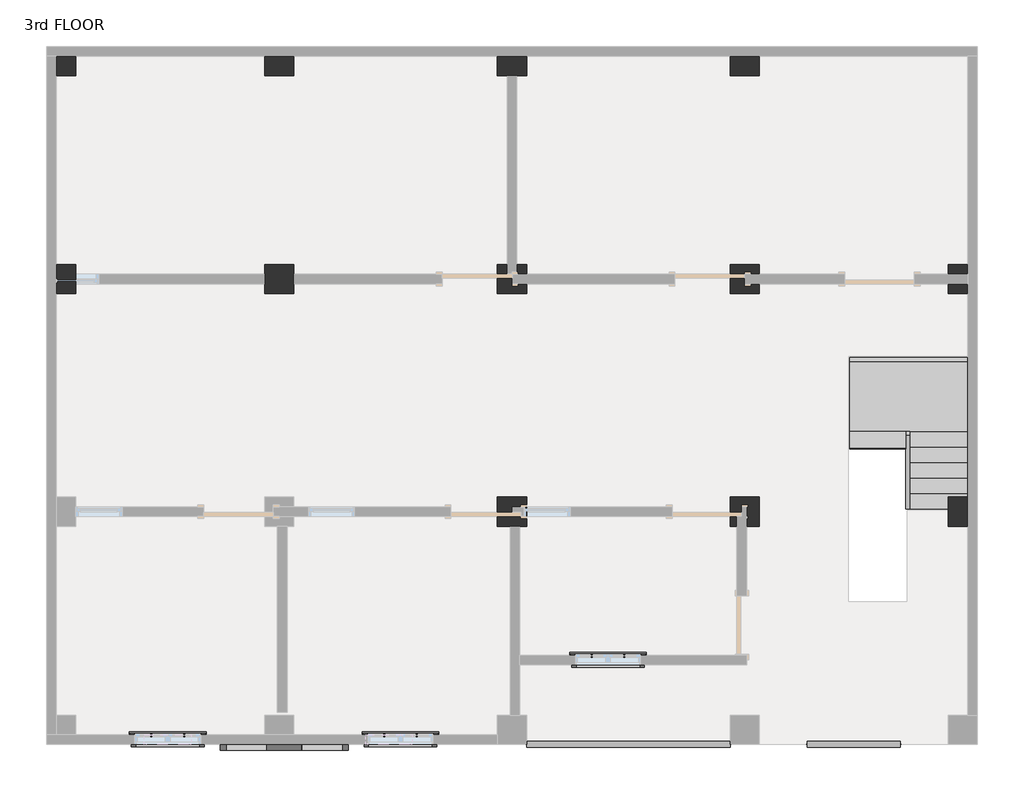
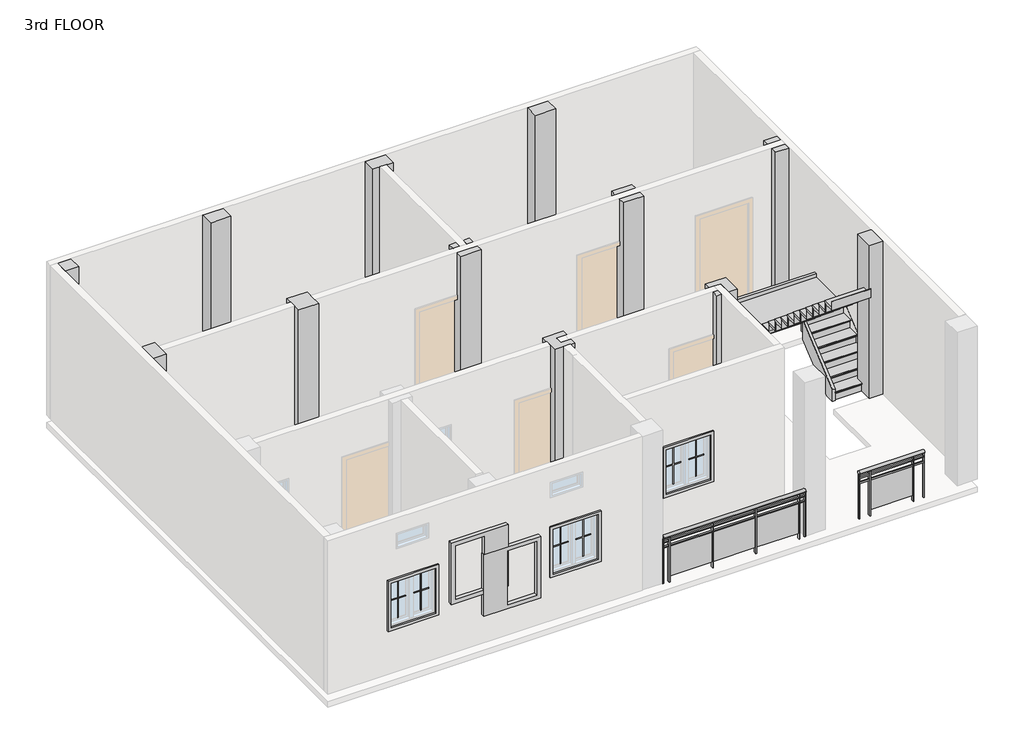
# One storey, part 2 of 2: 12 columns, 12 proxies, 4 members, 2 railings, 1 damper, 1 stair flight.
"""IFC4 building model written with IfcOpenShell, lengths in millimetres."""

from ifc_helpers import new_model, si_unit, point, frame, origin, place, context, project, spatial, polyline, ellipse_curve, trimmed, outline, extrude, faceted_brep, transform, mapped, element, save
from ifc_brep_helpers import plane_surface, extruded_surface, advanced_brep
from components import muntin_pattern_2x2_muntin_pattern_2x2_b3fe6957, muntin_pattern_2x2_muntin_pattern_2x2_3e0ecaf2, trim_window_exterior_flat_with_sill_41619996, trim_window_interior_flat_picture_frame_51c85655, duct_accessories_10_duct_accessories_1_d43a2bea, stair_flight_e13e2030

model = new_model("IFC4")

# Units and contexts
model_context = context("Model", 3, world=origin())
ifc_project = project(units=[si_unit("LENGTHUNIT", "METRE", prefix="MILLI")], contexts=[model_context])

# Site, building, storey
site = spatial("IfcSite", under=ifc_project)
building = spatial("IfcBuilding", under=site)
storey = spatial("IfcBuildingStorey", under=building, Name="3rd FLOOR", Elevation=8991.6)

# Proxies
placement = place(None, origin())
muntin_pattern_2x2_muntin_pattern_2x2_shape = muntin_pattern_2x2_muntin_pattern_2x2_b3fe6957(model_context)
element("IfcBuildingElementProxy", 1, Name="Muntin Pattern_2x2 : Muntin Pattern_2x2", ObjectType="Muntin Pattern_2x2 : Muntin Pattern_2x2", at=placement, inside=storey, context=model_context, shape_type="MappedRepresentation", body=[
    mapped(muntin_pattern_2x2_muntin_pattern_2x2_shape, transform((-14441.409625, -253.8184478, 9975.85), x_axis=(1.0, 0.0, 0.0), y_axis=(0.0, 1.0, 0.0), z_axis=(0.0, 0.0, 1.0))),
])
element("IfcBuildingElementProxy", 2, Name="Muntin Pattern_2x2 : Muntin Pattern_2x2", ObjectType="Muntin Pattern_2x2 : Muntin Pattern_2x2", at=placement, inside=storey, context=model_context, shape_type="MappedRepresentation", body=[
    mapped(muntin_pattern_2x2_muntin_pattern_2x2_shape, transform((-11393.409625, -253.8184478, 9975.85), x_axis=(1.0, 0.0, 0.0), y_axis=(0.0, 1.0, 0.0), z_axis=(0.0, 0.0, 1.0))),
])
element("IfcBuildingElementProxy", 3, Name="Muntin Pattern_2x2 : Muntin Pattern_2x2", ObjectType="Muntin Pattern_2x2 : Muntin Pattern_2x2", at=placement, inside=storey, context=model_context, shape_type="MappedRepresentation", body=[
    mapped(muntin_pattern_2x2_muntin_pattern_2x2_shape, transform((-8675.609625, 787.5815522, 9975.85), x_axis=(1.0, 0.0, 0.0), y_axis=(0.0, 1.0, 0.0), z_axis=(0.0, 0.0, 1.0))),
])
muntin_pattern_2x2_muntin_pattern_2x2_2_shape = muntin_pattern_2x2_muntin_pattern_2x2_3e0ecaf2(model_context)
element("IfcBuildingElementProxy", 4, Name="Muntin Pattern_2x2 : Muntin Pattern_2x2", ObjectType="Muntin Pattern_2x2 : Muntin Pattern_2x2", at=placement, inside=storey, context=model_context, shape_type="MappedRepresentation", body=[
    mapped(muntin_pattern_2x2_muntin_pattern_2x2_2_shape, transform((-14012.784625, -253.8184478, 9975.85), x_axis=(-1.0, 0.0, 0.0), y_axis=(0.0, -1.0, 0.0), z_axis=(0.0, 0.0, 1.0))),
])
element("IfcBuildingElementProxy", 5, Name="Muntin Pattern_2x2 : Muntin Pattern_2x2", ObjectType="Muntin Pattern_2x2 : Muntin Pattern_2x2", at=placement, inside=storey, context=model_context, shape_type="MappedRepresentation", body=[
    mapped(muntin_pattern_2x2_muntin_pattern_2x2_2_shape, transform((-10964.784625, -253.8184478, 9975.85), x_axis=(-1.0, 0.0, 0.0), y_axis=(0.0, -1.0, 0.0), z_axis=(0.0, 0.0, 1.0))),
])
element("IfcBuildingElementProxy", 6, Name="Muntin Pattern_2x2 : Muntin Pattern_2x2", ObjectType="Muntin Pattern_2x2 : Muntin Pattern_2x2", at=placement, inside=storey, context=model_context, shape_type="MappedRepresentation", body=[
    mapped(muntin_pattern_2x2_muntin_pattern_2x2_2_shape, transform((-8246.984625, 787.5815522, 9975.85), x_axis=(-1.0, 0.0, 0.0), y_axis=(0.0, -1.0, 0.0), z_axis=(0.0, 0.0, 1.0))),
])
trim_window_exterior_flat_with_sill_shape = trim_window_exterior_flat_with_sill_41619996(model_context)
element("IfcBuildingElementProxy", 7, Name="Trim-Window-Exterior-Flat : with Sill", ObjectType="Trim-Window-Exterior-Flat : with Sill", at=placement, inside=storey, context=model_context, shape_type="MappedRepresentation", body=[
    mapped(trim_window_exterior_flat_with_sill_shape, transform((-14227.097125, -244.2934478, 10820.4), x_axis=(-1.0, 0.0, 0.0), y_axis=(0.0, 0.0, 1.0), z_axis=(0.0, 1.0, 0.0))),
])
element("IfcBuildingElementProxy", 8, Name="Trim-Window-Exterior-Flat : with Sill", ObjectType="Trim-Window-Exterior-Flat : with Sill", at=placement, inside=storey, context=model_context, shape_type="MappedRepresentation", body=[
    mapped(trim_window_exterior_flat_with_sill_shape, transform((-11179.097125, -244.2934478, 10820.4), x_axis=(-1.0, 0.0, 0.0), y_axis=(0.0, 0.0, 1.0), z_axis=(0.0, 1.0, 0.0))),
])
element("IfcBuildingElementProxy", 9, Name="Trim-Window-Exterior-Flat : with Sill", ObjectType="Trim-Window-Exterior-Flat : with Sill", at=placement, inside=storey, context=model_context, shape_type="MappedRepresentation", body=[
    mapped(trim_window_exterior_flat_with_sill_shape, transform((-8461.297125, 797.1065522, 10820.4), x_axis=(-1.0, 0.0, 0.0), y_axis=(0.0, 0.0, 1.0), z_axis=(0.0, 1.0, 0.0))),
])
trim_window_interior_flat_picture_frame_shape = trim_window_interior_flat_picture_frame_51c85655(model_context)
element("IfcBuildingElementProxy", 10, Name="Trim-Window-Interior-Flat : Picture Frame", ObjectType="Trim-Window-Interior-Flat : Picture Frame", at=placement, inside=storey, context=model_context, shape_type="MappedRepresentation", body=[
    mapped(trim_window_interior_flat_picture_frame_shape, transform((-14227.097125, -371.2934478, 10820.4), x_axis=(1.0, 0.0, 0.0), y_axis=(0.0, 0.0, 1.0), z_axis=(0.0, -1.0, 0.0))),
])
element("IfcBuildingElementProxy", 11, Name="Trim-Window-Interior-Flat : Picture Frame", ObjectType="Trim-Window-Interior-Flat : Picture Frame", at=placement, inside=storey, context=model_context, shape_type="MappedRepresentation", body=[
    mapped(trim_window_interior_flat_picture_frame_shape, transform((-11179.097125, -371.2934478, 10820.4), x_axis=(1.0, 0.0, 0.0), y_axis=(0.0, 0.0, 1.0), z_axis=(0.0, -1.0, 0.0))),
])
element("IfcBuildingElementProxy", 12, Name="Trim-Window-Interior-Flat : Picture Frame", ObjectType="Trim-Window-Interior-Flat : Picture Frame", at=placement, inside=storey, context=model_context, shape_type="MappedRepresentation", body=[
    mapped(trim_window_interior_flat_picture_frame_shape, transform((-8461.297125, 670.1065522, 10820.4), x_axis=(1.0, 0.0, 0.0), y_axis=(0.0, 0.0, 1.0), z_axis=(0.0, -1.0, 0.0))),
])

# Columns
element("IfcColumn", 13, ObjectType="column family : column family", at=placement, inside=storey, context=model_context, shape_type="SweptSolid", body=[
    extrude(outline(polyline([(-15433.597125, 8645.7065522), (-15433.597125, 8391.7065522), (-15687.597125, 8391.7065522), (-15687.597125, 8645.7065522), (-15433.597125, 8645.7065522)])), frame((0.0, 0.0, 8996.6), z_axis=(0.0, 0.0, 1.0), x_axis=(1.0, 0.0, 0.0)), (0.0, 0.0, 1.0), 3038.0),
])
element("IfcColumn", 14, ObjectType="column family : column family", at=placement, inside=storey, context=model_context, shape_type="SweptSolid", body=[
    extrude(outline(polyline([(-12576.097125, 5915.2065522), (-12576.097125, 5534.2065522), (-12957.097125, 5534.2065522), (-12957.097125, 5915.2065522), (-12576.097125, 5915.2065522)])), frame((0.0, 0.0, 8996.6), z_axis=(0.0, 0.0, 1.0), x_axis=(1.0, 0.0, 0.0)), (0.0, 0.0, 1.0), 3038.0),
])
element("IfcColumn", 15, ObjectType="column family : column family", at=placement, inside=storey, context=model_context, shape_type="Brep", body=[
    faceted_brep([(-9655.097125, 5915.2065522, 8996.6), (-9528.097125, 5915.2065522, 8996.6), (-9528.097125, 5788.2065522, 8996.6), (-9655.097125, 5788.2065522, 8996.6), (-9528.097125, 5915.2065522, 12034.6), (-9655.097125, 5915.2065522, 12034.6), (-9655.097125, 5788.2065522, 12034.6), (-9528.097125, 5788.2065522, 12034.6)], [[[0, 1, 2, 3]], [[4, 5, 6, 7]], [[0, 3, 6, 5]], [[4, 1, 0, 5]], [[3, 2, 7, 6]], [[1, 4, 7, 2]]]),
    faceted_brep([(-9528.097125, 5534.2065522, 12034.6), (-9528.097125, 5534.2065522, 8996.6), (-9528.097125, 5661.2065522, 8996.6), (-9528.097125, 5661.2065522, 12034.6), (-9909.097125, 5534.2065522, 8996.6), (-9909.097125, 5534.2065522, 12034.6), (-9909.097125, 5915.2065522, 8996.6), (-9909.097125, 5661.2065522, 12034.6), (-9909.097125, 5661.2065522, 11125.2), (-9909.097125, 5788.2065522, 11125.2), (-9909.097125, 5788.2065522, 12034.6), (-9909.097125, 5915.2065522, 12034.6), (-9782.097125, 5915.2065522, 12034.6), (-9782.097125, 5915.2065522, 8996.6), (-9782.097125, 5788.2065522, 8996.6), (-9782.097125, 5788.2065522, 12034.6), (-9782.097125, 5788.2065522, 11125.2), (-9718.597125, 5788.2065522, 8996.6), (-9718.597125, 5788.2065522, 11125.2), (-9718.597125, 5661.2065522, 8996.6), (-9718.597125, 5661.2065522, 11125.2)], [[[0, 1, 2, 3]], [[4, 1, 0, 5]], [[6, 4, 5, 7, 8, 9, 10, 11]], [[6, 11, 12, 13]], [[14, 13, 12, 15, 16]], [[17, 14, 16, 18]], [[19, 20, 8, 7, 3, 2]], [[1, 4, 6, 13, 14, 17, 19, 2]], [[5, 0, 3, 7]], [[12, 11, 10, 15]], [[9, 16, 15, 10]], [[18, 20, 19, 17]], [[20, 18, 16, 9, 8]]]),
])
element("IfcColumn", 16, ObjectType="column family : column family", at=placement, inside=storey, context=model_context, shape_type="Brep", body=[
    faceted_brep([(-6480.097125, 5534.2065522, 8996.6), (-6861.097125, 5534.2065522, 8996.6), (-6861.097125, 5915.2065522, 8996.6), (-6480.097125, 5915.2065522, 8996.6), (-6480.097125, 5788.2065522, 8996.6), (-6670.597125, 5788.2065522, 8996.6), (-6670.597125, 5661.2065522, 8996.6), (-6480.097125, 5661.2065522, 8996.6), (-6480.097125, 5534.2065522, 12034.6), (-6480.097125, 5661.2065522, 12034.6), (-6861.097125, 5534.2065522, 12034.6), (-6861.097125, 5661.2065522, 12034.6), (-6861.097125, 5661.2065522, 11125.2), (-6861.097125, 5788.2065522, 11125.2), (-6861.097125, 5788.2065522, 12034.6), (-6861.097125, 5915.2065522, 12034.6), (-6480.097125, 5915.2065522, 12034.6), (-6670.597125, 5661.2065522, 11125.2), (-6670.597125, 5788.2065522, 11125.2), (-6480.097125, 5788.2065522, 12034.6)], [[[0, 1, 2, 3, 4, 5, 6, 7]], [[8, 0, 7, 9]], [[1, 0, 8, 10]], [[2, 1, 10, 11, 12, 13, 14, 15]], [[3, 2, 15, 16]], [[10, 8, 9, 11]], [[6, 17, 12, 11, 9, 7]], [[13, 18, 5, 4, 19, 14]], [[3, 16, 19, 4]], [[16, 15, 14, 19]], [[18, 17, 6, 5]], [[17, 18, 13, 12]]]),
])
element("IfcColumn", 17, ObjectType="column family : column family", at=placement, inside=storey, context=model_context, shape_type="Brep", body=[
    faceted_brep([(-6480.097125, 2867.2065522, 8996.6), (-6480.097125, 2486.2065522, 8996.6), (-6645.197125, 2486.2065522, 8996.6), (-6645.197125, 2740.2065522, 8996.6), (-6708.697125, 2740.2065522, 8996.6), (-6708.697125, 2613.2065522, 8996.6), (-6772.197125, 2613.2065522, 8996.6), (-6772.197125, 2486.2065522, 8996.6), (-6861.097125, 2486.2065522, 8996.6), (-6861.097125, 2867.2065522, 8996.6), (-6480.097125, 2867.2065522, 12034.6), (-6480.097125, 2486.2065522, 12034.6), (-6861.097125, 2486.2065522, 12034.6), (-6772.197125, 2486.2065522, 12034.6), (-6861.097125, 2613.2065522, 12034.6), (-6861.097125, 2613.2065522, 11125.2), (-6861.097125, 2740.2065522, 11125.2), (-6861.097125, 2740.2065522, 12034.6), (-6861.097125, 2867.2065522, 12034.6), (-6772.197125, 2740.2065522, 12034.6), (-6645.197125, 2740.2065522, 12034.6), (-6645.197125, 2486.2065522, 12034.6), (-6772.197125, 2613.2065522, 12034.6), (-6772.197125, 2613.2065522, 11125.2), (-6772.197125, 2740.2065522, 11125.2), (-6708.697125, 2613.2065522, 11125.2), (-6708.697125, 2740.2065522, 11125.2)], [[[0, 1, 2, 3, 4, 5, 6, 7, 8, 9]], [[1, 0, 10, 11]], [[12, 8, 7, 13]], [[9, 8, 12, 14, 15, 16, 17, 18]], [[0, 9, 18, 10]], [[11, 10, 18, 17, 19, 20, 21]], [[15, 14, 22, 23]], [[17, 16, 24, 19]], [[20, 3, 2, 21]], [[6, 23, 22, 13, 7]], [[14, 12, 13, 22]], [[1, 11, 21, 2]], [[15, 23, 24, 16]], [[25, 23, 6, 5]], [[23, 25, 26, 24]], [[26, 25, 5, 4]], [[24, 26, 4, 3, 20, 19]]]),
])
element("IfcColumn", 18, ObjectType="column family : column family", at=placement, inside=storey, context=model_context, shape_type="Brep", body=[
    faceted_brep([(-9528.097125, 2486.2065522, 8996.6), (-9909.097125, 2486.2065522, 8996.6), (-9909.097125, 2867.2065522, 8996.6), (-9528.097125, 2867.2065522, 8996.6), (-9528.097125, 2740.2065522, 8996.6), (-9566.197125, 2740.2065522, 8996.6), (-9718.597125, 2740.2065522, 8996.6), (-9718.597125, 2613.2065522, 8996.6), (-9566.197125, 2613.2065522, 8996.6), (-9528.097125, 2613.2065522, 8996.6), (-9528.097125, 2486.2065522, 12034.6), (-9528.097125, 2613.2065522, 9296.4), (-9528.097125, 2740.2065522, 9296.4), (-9528.097125, 2867.2065522, 12034.6), (-9528.097125, 2740.2065522, 12034.6), (-9528.097125, 2740.2065522, 11125.2), (-9528.097125, 2613.2065522, 11125.2), (-9528.097125, 2613.2065522, 12034.6), (-9909.097125, 2486.2065522, 12034.6), (-9909.097125, 2867.2065522, 12034.6), (-9566.197125, 2613.2065522, 12034.6), (-9718.597125, 2613.2065522, 12034.6), (-9718.597125, 2740.2065522, 12034.6), (-9566.197125, 2740.2065522, 12034.6), (-9566.197125, 2613.2065522, 11125.2), (-9566.197125, 2613.2065522, 9296.4), (-9566.197125, 2740.2065522, 9296.4), (-9566.197125, 2740.2065522, 11125.2)], [[[0, 1, 2, 3, 4, 5, 6, 7, 8, 9]], [[10, 0, 9, 11, 12, 4, 3, 13, 14, 15, 16, 17]], [[1, 0, 10, 18]], [[2, 1, 18, 19]], [[3, 2, 19, 13]], [[18, 10, 17, 20, 21, 22, 23, 14, 13, 19]], [[11, 9, 8, 7, 21, 20, 17, 16, 24, 25]], [[4, 12, 26, 27, 15, 14, 23, 22, 6, 5]], [[21, 7, 6, 22]], [[25, 24, 27, 26]], [[25, 26, 12, 11]], [[27, 24, 16, 15]]]),
])
element("IfcColumn", 19, ObjectType="column family : column family", at=placement, inside=storey, context=model_context, shape_type="SweptSolid", body=[
    extrude(outline(polyline([(-12576.097125, 8391.7065522), (-12957.097125, 8391.7065522), (-12957.097125, 8645.7065522), (-12576.097125, 8645.7065522), (-12576.097125, 8391.7065522)])), frame((0.0, 0.0, 8996.6), z_axis=(0.0, 0.0, 1.0), x_axis=(1.0, 0.0, 0.0)), (0.0, 0.0, 1.0), 3038.0),
])
element("IfcColumn", 20, ObjectType="column family : column family", at=placement, inside=storey, context=model_context, shape_type="SweptSolid", body=[
    extrude(outline(polyline([(-9528.097125, 8391.7065522), (-9909.097125, 8391.7065522), (-9909.097125, 8645.7065522), (-9528.097125, 8645.7065522), (-9528.097125, 8391.7065522)])), frame((0.0, 0.0, 8996.6), z_axis=(0.0, 0.0, 1.0), x_axis=(1.0, 0.0, 0.0)), (0.0, 0.0, 1.0), 3038.0),
])
element("IfcColumn", 21, ObjectType="column family : column family", at=placement, inside=storey, context=model_context, shape_type="SweptSolid", body=[
    extrude(outline(polyline([(-6480.097125, 8391.7065522), (-6861.097125, 8391.7065522), (-6861.097125, 8645.7065522), (-6480.097125, 8645.7065522), (-6480.097125, 8391.7065522)])), frame((0.0, 0.0, 8996.6), z_axis=(0.0, 0.0, 1.0), x_axis=(1.0, 0.0, 0.0)), (0.0, 0.0, 1.0), 3038.0),
])
element("IfcColumn", 22, ObjectType="column family : column family", at=placement, inside=storey, context=model_context, shape_type="SweptSolid", body=[
    extrude(outline(polyline([(-4003.597125, 5915.2065522), (-3749.597125, 5915.2065522), (-3749.597125, 5788.2065522), (-4003.597125, 5788.2065522), (-4003.597125, 5915.2065522)])), frame((0.0, 0.0, 8996.6), z_axis=(0.0, 0.0, 1.0), x_axis=(1.0, 0.0, 0.0)), (0.0, 0.0, 1.0), 3038.0),
    extrude(outline(polyline([(-3749.597125, 5534.2065522), (-4003.597125, 5534.2065522), (-4003.597125, 5661.2065522), (-3749.597125, 5661.2065522), (-3749.597125, 5534.2065522)])), frame((0.0, 0.0, 8996.6), z_axis=(0.0, 0.0, 1.0), x_axis=(1.0, 0.0, 0.0)), (0.0, 0.0, 1.0), 3038.0),
])
element("IfcColumn", 23, ObjectType="column family : column family", at=placement, inside=storey, context=model_context, shape_type="SweptSolid", body=[
    extrude(outline(polyline([(-4003.597125, 2486.2065522), (-4003.597125, 2867.2065522), (-3749.597125, 2867.2065522), (-3749.597125, 2486.2065522), (-4003.597125, 2486.2065522)])), frame((0.0, 0.0, 8996.6), z_axis=(0.0, 0.0, 1.0), x_axis=(1.0, 0.0, 0.0)), (0.0, 0.0, 1.0), 3038.0),
])
element("IfcColumn", 24, ObjectType="column family : column family", at=placement, inside=storey, context=model_context, shape_type="SweptSolid", body=[
    extrude(outline(polyline([(-15433.597125, 5915.2065522), (-15433.597125, 5534.2065522), (-15687.597125, 5534.2065522), (-15687.597125, 5915.2065522), (-15433.597125, 5915.2065522)])), frame((0.0, 0.0, 8996.6), z_axis=(0.0, 0.0, 1.0), x_axis=(1.0, 0.0, 0.0)), (0.0, 0.0, 1.0), 3038.0),
])

# Damper
duct_accessories_10_duct_accessories_1_shape = duct_accessories_10_duct_accessories_1_d43a2bea(model_context)
element("IfcDamper", 25, ObjectType="Duct Accessories 10 : Duct Accessories 1", at=placement, inside=storey, context=model_context, shape_type="MappedRepresentation", body=[
    mapped(duct_accessories_10_duct_accessories_1_shape, transform((0.0, 0.0, 0.0), x_axis=(1.0, 0.0, 0.0), y_axis=(0.0, 1.0, 0.0), z_axis=(0.0, 0.0, 1.0))),
])

# Members
element("IfcMember", 26, ObjectType="Stringer - 2\" Width", at=placement, inside=storey, context=model_context, shape_type="SweptSolid", body=[
    extrude(outline(polyline([(2714.6319226, 8991.6), (2714.6319226, 9228.4438745), (3679.8319226, 10032.7772078), (3679.8319226, 9636.0165243), (2906.5320935, 8991.6), (2714.6319226, 8991.6)])), frame((-4563.0136682, 0.0, 0.0), z_axis=(1.0, 0.0, 0.0), x_axis=(0.0, 1.0, 0.0)), (0.0, 0.0, 1.0), 50.8),
])
element("IfcMember", 27, ObjectType="Stringer - 2\" Width", at=placement, inside=storey, context=model_context, shape_type="SweptSolid", body=[
    extrude(outline(polyline([(-4512.2136682, 3730.6319226), (-4512.2136682, 3679.8319226), (-4563.0136682, 3679.8319226), (-4563.0136682, 3730.6319226), (-4512.2136682, 3730.6319226)])), frame((0.0, 0.0, 9779.0), z_axis=(0.0, 0.0, 1.0), x_axis=(1.0, 0.0, 0.0)), (0.0, 0.0, 1.0), 304.8),
])
element("IfcMember", 28, ObjectType="Stringer - 2\" Width", at=placement, inside=storey, context=model_context, shape_type="SweptSolid", body=[
    extrude(outline(polyline([(2714.6319226, 8991.6), (2714.6319226, 9228.4438745), (3741.0592732, 10083.8), (4217.1720935, 10083.8), (2906.5320935, 8991.6), (2714.6319226, 8991.6)])), frame((-3749.597125, 0.0, 0.0), z_axis=(1.0, 0.0, 0.0), x_axis=(0.0, 1.0, 0.0)), (0.0, 0.0, 1.0), 50.8),
])
element("IfcMember", 29, ObjectType="Stringer - 2\" Width", at=placement, inside=storey, context=model_context, shape_type="SweptSolid", body=[
    extrude(outline(polyline([(-3698.797125, 4695.8319226), (-3698.797125, 4645.0319226), (-5295.0246464, 4645.0319226), (-5295.0246464, 4695.8319226), (-3698.797125, 4695.8319226)])), frame((0.0, 0.0, 9779.0), z_axis=(0.0, 0.0, 1.0), x_axis=(1.0, 0.0, 0.0)), (0.0, 0.0, 1.0), 304.8),
])

# Railings
element("IfcRailing", 30, ObjectType="Glass Panel - Bottom Fill", at=placement, inside=storey, context=model_context, shape_type="SolidModel", body=[
    advanced_brep(
    [(-9528.097125, -333.1934478, 9906.0), (-9528.097125, -409.3934478, 9906.0), (-6861.097125, -333.1934478, 9906.0), (-6861.097125, -409.3934478, 9906.0)],
    [
        (0, 1, ellipse_curve(frame((-9528.097125, -371.2934478, 9906.0), z_axis=(-1.0, 0.0, 0.0), x_axis=(0.0, -1.0, 0.0)), 38.1, 28.575)),
        (1, 0, ellipse_curve(frame((-9528.097125, -371.2934478, 9906.0), z_axis=(-1.0, 0.0, 0.0), x_axis=(0.0, -1.0, 0.0)), 38.1, 28.575)),
        (2, 3, ellipse_curve(frame((-6861.097125, -371.2934478, 9906.0), z_axis=(1.0, 0.0, 0.0), x_axis=(0.0, -1.0, 0.0)), 38.1, 28.575)),
        (3, 2, ellipse_curve(frame((-6861.097125, -371.2934478, 9906.0), z_axis=(1.0, 0.0, 0.0), x_axis=(0.0, -1.0, 0.0)), 38.1, 28.575)),
        (0, 2),
        (3, 1),
    ],
    [
        plane_surface(frame((-9528.097125, -371.2934478, 9906.0), z_axis=(-1.0, 0.0, 0.0), x_axis=(0.0, 1.0, 0.0))),
        plane_surface(frame((-6861.097125, -371.2934478, 9906.0), z_axis=(1.0, 0.0, 0.0), x_axis=(0.0, 1.0, 0.0))),
        extruded_surface(trimmed(ellipse_curve(frame((-6861.097125, -371.2934478, 9906.0), z_axis=(-1.0, 0.0, 0.0), x_axis=(0.0, -1.0, 0.0)), 38.1, 28.575), [point((-6861.097125, -333.1934478, 9906.0))], [point((-6861.097125, -409.3934478, 9906.0))], True, "CARTESIAN"), (-2667.0, 0.0, 0.0), 2667.0),
        extruded_surface(trimmed(ellipse_curve(frame((-6861.097125, -371.2934478, 9906.0), z_axis=(-1.0, 0.0, 0.0), x_axis=(0.0, -1.0, 0.0)), 38.1, 28.575), [point((-6861.097125, -409.3934478, 9906.0))], [point((-6861.097125, -333.1934478, 9906.0))], True, "CARTESIAN"), (-2667.0, 0.0, 0.0), 2667.0),
    ],
    [
        (0, [[1, 2]]),
        (1, [[3, 4]]),
        (2, [[-1, 5, -4, 6]]),
        (3, [[-2, -6, -3, -5]]),
    ],
),
    extrude(outline(polyline([(-9528.097125, -383.9934478), (-9528.097125, -358.5934478), (-6861.097125, -358.5934478), (-6861.097125, -383.9934478), (-9528.097125, -383.9934478)])), frame((0.0, 0.0, 9791.7), z_axis=(0.0, 0.0, 1.0), x_axis=(1.0, 0.0, 0.0)), (0.0, 0.0, 1.0), 25.4),
    extrude(outline(polyline([(-9528.097125, -383.9934478), (-9528.097125, -358.5934478), (-6861.097125, -358.5934478), (-6861.097125, -383.9934478), (-9528.097125, -383.9934478)])), frame((0.0, 0.0, 9690.1), z_axis=(0.0, 0.0, 1.0), x_axis=(1.0, 0.0, 0.0)), (0.0, 0.0, 1.0), 25.4),
    extrude(outline(polyline([(-6981.747125, -396.6934478), (-6981.747125, -345.8934478), (-6969.047125, -345.8934478), (-6969.047125, -396.6934478), (-6981.747125, -396.6934478)])), frame((0.0, 0.0, 8991.6), z_axis=(0.0, 0.0, 1.0), x_axis=(1.0, 0.0, 0.0)), (0.0, 0.0, 1.0), 885.6788223),
    extrude(outline(polyline([(-7788.197125, -364.7582908), (-6975.397125, -364.7582908), (-6975.397125, -371.1082908), (-7788.197125, -371.1082908), (-7788.197125, -364.7582908)])), frame((0.0, 0.0, 9093.2), z_axis=(0.0, 0.0, 1.0), x_axis=(1.0, 0.0, 0.0)), (0.0, 0.0, 1.0), 596.9),
    extrude(outline(polyline([(-7794.547125, -396.6934478), (-7794.547125, -345.8934478), (-7781.847125, -345.8934478), (-7781.847125, -396.6934478), (-7794.547125, -396.6934478)])), frame((0.0, 0.0, 8991.6), z_axis=(0.0, 0.0, 1.0), x_axis=(1.0, 0.0, 0.0)), (0.0, 0.0, 1.0), 885.6788223),
    extrude(outline(polyline([(-8600.997125, -364.7582908), (-7788.197125, -364.7582908), (-7788.197125, -371.1082908), (-8600.997125, -371.1082908), (-8600.997125, -364.7582908)])), frame((0.0, 0.0, 9093.2), z_axis=(0.0, 0.0, 1.0), x_axis=(1.0, 0.0, 0.0)), (0.0, 0.0, 1.0), 596.9),
    extrude(outline(polyline([(-8607.347125, -396.6934478), (-8607.347125, -345.8934478), (-8594.647125, -345.8934478), (-8594.647125, -396.6934478), (-8607.347125, -396.6934478)])), frame((0.0, 0.0, 8991.6), z_axis=(0.0, 0.0, 1.0), x_axis=(1.0, 0.0, 0.0)), (0.0, 0.0, 1.0), 885.6788223),
    extrude(outline(polyline([(-9413.797125, -364.7582908), (-8600.997125, -364.7582908), (-8600.997125, -371.1082908), (-9413.797125, -371.1082908), (-9413.797125, -364.7582908)])), frame((0.0, 0.0, 9093.2), z_axis=(0.0, 0.0, 1.0), x_axis=(1.0, 0.0, 0.0)), (0.0, 0.0, 1.0), 596.9),
    extrude(outline(polyline([(-9420.147125, -396.6934478), (-9420.147125, -345.8934478), (-9407.447125, -345.8934478), (-9407.447125, -396.6934478), (-9420.147125, -396.6934478)])), frame((0.0, 0.0, 8991.6), z_axis=(0.0, 0.0, 1.0), x_axis=(1.0, 0.0, 0.0)), (0.0, 0.0, 1.0), 885.6788223),
    extrude(outline(polyline([(-6873.797125, -380.8184478), (-6873.797125, -361.7684478), (-6854.747125, -361.7684478), (-6854.747125, -380.8184478), (-6873.797125, -380.8184478)])), frame((0.0, 0.0, 8991.6), z_axis=(0.0, 0.0, 1.0), x_axis=(1.0, 0.0, 0.0)), (0.0, 0.0, 1.0), 885.6788223),
    extrude(outline(polyline([(-9534.447125, -380.8184478), (-9534.447125, -361.7684478), (-9515.397125, -361.7684478), (-9515.397125, -380.8184478), (-9534.447125, -380.8184478)])), frame((0.0, 0.0, 8991.6), z_axis=(0.0, 0.0, 1.0), x_axis=(1.0, 0.0, 0.0)), (0.0, 0.0, 1.0), 885.6788223),
])
element("IfcRailing", 31, ObjectType="Glass Panel - Bottom Fill", at=placement, inside=storey, context=model_context, shape_type="SolidModel", body=[
    advanced_brep(
    [(-5851.447125, -333.1934478, 9906.0), (-5851.447125, -409.3934478, 9906.0), (-4632.247125, -333.1934478, 9906.0), (-4632.247125, -409.3934478, 9906.0)],
    [
        (0, 1, ellipse_curve(frame((-5851.447125, -371.2934478, 9906.0), z_axis=(-1.0, 0.0, 0.0), x_axis=(0.0, -1.0, 0.0)), 38.1, 28.575)),
        (1, 0, ellipse_curve(frame((-5851.447125, -371.2934478, 9906.0), z_axis=(-1.0, 0.0, 0.0), x_axis=(0.0, -1.0, 0.0)), 38.1, 28.575)),
        (2, 3, ellipse_curve(frame((-4632.247125, -371.2934478, 9906.0), z_axis=(1.0, 0.0, 0.0), x_axis=(0.0, -1.0, 0.0)), 38.1, 28.575)),
        (3, 2, ellipse_curve(frame((-4632.247125, -371.2934478, 9906.0), z_axis=(1.0, 0.0, 0.0), x_axis=(0.0, -1.0, 0.0)), 38.1, 28.575)),
        (0, 2),
        (3, 1),
    ],
    [
        plane_surface(frame((-5851.447125, -371.2934478, 9906.0), z_axis=(-1.0, 0.0, 0.0), x_axis=(0.0, 1.0, 0.0))),
        plane_surface(frame((-4632.247125, -371.2934478, 9906.0), z_axis=(1.0, 0.0, 0.0), x_axis=(0.0, 1.0, 0.0))),
        extruded_surface(trimmed(ellipse_curve(frame((-4632.247125, -371.2934478, 9906.0), z_axis=(-1.0, 0.0, 0.0), x_axis=(0.0, -1.0, 0.0)), 38.1, 28.575), [point((-4632.247125, -333.1934478, 9906.0))], [point((-4632.247125, -409.3934478, 9906.0))], True, "CARTESIAN"), (-1219.1999999999998, 0.0, 0.0), 1219.1999999999998),
        extruded_surface(trimmed(ellipse_curve(frame((-4632.247125, -371.2934478, 9906.0), z_axis=(-1.0, 0.0, 0.0), x_axis=(0.0, -1.0, 0.0)), 38.1, 28.575), [point((-4632.247125, -409.3934478, 9906.0))], [point((-4632.247125, -333.1934478, 9906.0))], True, "CARTESIAN"), (-1219.1999999999998, 0.0, 0.0), 1219.1999999999998),
    ],
    [
        (0, [[1, 2]]),
        (1, [[3, 4]]),
        (2, [[-1, 5, -4, 6]]),
        (3, [[-2, -6, -3, -5]]),
    ],
),
    extrude(outline(polyline([(-5851.447125, -383.9934478), (-5851.447125, -358.5934478), (-4632.247125, -358.5934478), (-4632.247125, -383.9934478), (-5851.447125, -383.9934478)])), frame((0.0, 0.0, 9791.7), z_axis=(0.0, 0.0, 1.0), x_axis=(1.0, 0.0, 0.0)), (0.0, 0.0, 1.0), 25.4),
    extrude(outline(polyline([(-5851.447125, -383.9934478), (-5851.447125, -358.5934478), (-4632.247125, -358.5934478), (-4632.247125, -383.9934478), (-5851.447125, -383.9934478)])), frame((0.0, 0.0, 9690.1), z_axis=(0.0, 0.0, 1.0), x_axis=(1.0, 0.0, 0.0)), (0.0, 0.0, 1.0), 25.4),
    extrude(outline(polyline([(-4841.797125, -396.6934478), (-4841.797125, -345.8934478), (-4829.097125, -345.8934478), (-4829.097125, -396.6934478), (-4841.797125, -396.6934478)])), frame((0.0, 0.0, 8991.6), z_axis=(0.0, 0.0, 1.0), x_axis=(1.0, 0.0, 0.0)), (0.0, 0.0, 1.0), 885.6788223),
    extrude(outline(polyline([(-5648.247125, -364.7582908), (-4835.447125, -364.7582908), (-4835.447125, -371.1082908), (-5648.247125, -371.1082908), (-5648.247125, -364.7582908)])), frame((0.0, 0.0, 9093.2), z_axis=(0.0, 0.0, 1.0), x_axis=(1.0, 0.0, 0.0)), (0.0, 0.0, 1.0), 596.9),
    extrude(outline(polyline([(-5654.597125, -396.6934478), (-5654.597125, -345.8934478), (-5641.897125, -345.8934478), (-5641.897125, -396.6934478), (-5654.597125, -396.6934478)])), frame((0.0, 0.0, 8991.6), z_axis=(0.0, 0.0, 1.0), x_axis=(1.0, 0.0, 0.0)), (0.0, 0.0, 1.0), 885.6788223),
    extrude(outline(polyline([(-4644.947125, -380.8184478), (-4644.947125, -361.7684478), (-4625.897125, -361.7684478), (-4625.897125, -380.8184478), (-4644.947125, -380.8184478)])), frame((0.0, 0.0, 8991.6), z_axis=(0.0, 0.0, 1.0), x_axis=(1.0, 0.0, 0.0)), (0.0, 0.0, 1.0), 885.6788223),
    extrude(outline(polyline([(-5857.797125, -380.8184478), (-5857.797125, -361.7684478), (-5838.747125, -361.7684478), (-5838.747125, -380.8184478), (-5857.797125, -380.8184478)])), frame((0.0, 0.0, 8991.6), z_axis=(0.0, 0.0, 1.0), x_axis=(1.0, 0.0, 0.0)), (0.0, 0.0, 1.0), 885.6788223),
])

# Stair flight
stair_flight_shape = stair_flight_e13e2030(model_context)
element("IfcStairFlight", 32, ObjectType="2\" Tread 1\" Nosing 1/4\" Riser", at=placement, inside=storey, context=model_context, shape_type="MappedRepresentation", body=[
    mapped(stair_flight_shape, transform((0.0, 0.0, 0.0), x_axis=(1.0, 0.0, 0.0), y_axis=(0.0, 1.0, 0.0), z_axis=(0.0, 0.0, 1.0))),
])

save(model, "model.ifc")

# Revit data of these elements
# Type "Muntin Pattern_2x2 : Muntin Pattern_2x2"
#   Width [instance default] = 4' - 0"
#   Thickness = 0' - 0 1/2"
#   Height [instance default] = 4' - 0"
#   Distance = 0' - 0 3/4"
#   Interior Material [instance default] = none
#   Exterior Material [instance default] = none
#   Default Elevation = 0
# Type "Trim-Window-Exterior-Flat : with Sill"
#   Trim Width = 0' - 2 1/4"
#   Trim Thickness_Picture Frame = 0' - 1 1/4"
#   Trim Thickness_with Sill = 0' - 0 3/4"
#   Sill Thickness = 0' - 1 1/4"
#   Opening Width [instance default] = 2' - 0"
#   Opening Height [instance default] = 3' - 0"
#   Default Elevation = 4' - 0"
#   Sill = yes
#   Picture Frame = no
#   Trim Material [instance default] = none
# Type "Trim-Window-Interior-Flat : Picture Frame"
#   Trim Thickness_Picture Frame = 0' - 1 1/4"
#   Trim Width = 0' - 2 1/4"
#   Trim Thickness_with Sill = 0' - 0 3/4"
#   Sill Thickness = 0' - 1 1/4"
#   Opening Width [instance default] = 2' - 0"
#   Opening Height [instance default] = 3' - 0"
#   Default Elevation = 4' - 0"
#   Sill = no
#   Picture Frame = yes
#   Trim Material [instance default] = none
# Type "column family : column family"
#   w2 [instance default] = 0' - 9.88189"
#   w1 [instance default] = 0' - 9.01575"
#   Depth = 1' - 11.62205"
#   Width = 1' - 11.62205"
# Type "Glass Panel - Bottom Fill"
#   Assembly Code = "C2010400"
#   built-in parameter 1008612 = 0.0416667 (stored number, unit not read)
#   built-in parameter 1008611 = 0.0416667 (stored number, unit not read)
#   built-in parameter 1008609 = 0.333333 (stored number, unit not read)
#   built-in parameter 1008604 = 0.166667 (stored number, unit not read)
#   built-in parameter 1008603 = 0.166667 (stored number, unit not read)
#   Railing Height = 3' - 0"
#   built-in parameter 1008630 = 2
#   built-in parameter 1008610 = 2
#   built-in parameter 1008618 = Baluster - Square : 3/4"
# Elements 1, 2, 3, 4, 5, 6 (IfcBuildingElementProxy, "Muntin Pattern_2x2 : Muntin Pattern_2x2")
#   Width = 0' - 11 5/8"
#   Height = 2' - 6 1/2"
#   Interior Material = Wood - Stained
#   Exterior Material = Clad - White
#   Phase Created = New Construction
#   Materials on its faces: "Clad - White", "Wood - Stained"
# Elements 7, 8, 9 (IfcBuildingElementProxy, "Trim-Window-Exterior-Flat : with Sill")
#   Opening Width = 2' - 10"
#   Opening Height = 3' - 0"
#   Trim Material = Clad - White
#   Phase Created = New Construction
#   Materials on its faces: "Clad - White"
# Elements 10, 11, 12 (IfcBuildingElementProxy, "Trim-Window-Interior-Flat : Picture Frame")
#   Opening Width = 2' - 10"
#   Opening Height = 3' - 0"
#   Trim Material = Wood - Stained
#   Phase Created = New Construction
#   Materials on its faces: "Wood - Stained"
# Elements 13, 14, 15, 19, 20, 21 (IfcColumn, "column family : column family")
#   w2 = 1' - 3"
#   w1 = 1' - 3"
#   Phase Created = New Construction
#   Materials on its faces: "Default Wall"
# Elements 16, 22, 23 (IfcColumn, "column family : column family")
#   w2 = 1' - 3"
#   w1 = 1' - 3"
#   Phase Created = New Construction
#   Materials on its faces: "grey", "Default Wall"
# Elements 17, 18 (IfcColumn, "column family : column family")
#   w2 = 1' - 3"
#   w1 = 1' - 3"
#   Phase Created = New Construction
#   Materials on its faces: "Default Wall", "inside wall"
# Element 24 (IfcColumn, "column family : column family")
#   w2 = 1' - 3"
#   w1 = 1' - 3"
#   Phase Created = New Construction
#   Materials on its faces: "inside wall", "Default Wall"
# Element 25 (IfcDamper, "Duct Accessories 10 : Duct Accessories 1")
#   Mark = "10"
#   Phase Created = New Construction
#   Materials on its faces: "border"
# Elements 26, 27, 28, 29 (IfcMember, "Stringer - 2\" Width")
#   Phase Created = New Construction
# Elements 30, 31 (IfcRailing, "Glass Panel - Bottom Fill")
#   Phase Created = New Construction
#   Materials on its faces: "Glass"
# Element 32 (IfcStairFlight, "2\" Tread 1\" Nosing 1/4\" Riser")
#   Phase Created = New Construction
# Materials
#   "Clad - White": class "Wood", colour RGB 242 242 238, transparency 0, Cost = 0
#   "Wood - Stained": class "Wood", colour RGB 224 178 126, transparency 0, Cost = 0
#   "Default Wall": colour RGB 128 128 128, transparency 0, Cost = 0
#   "grey": class "Generic", colour RGB 80 80 80, transparency 0, Cost = 0
#   "inside wall": class "Generic", colour RGB 199 224 95, transparency 0, Cost = 0
#   "border": class "Generic", colour RGB 144 144 144, transparency 0, Cost = 0
#   "Glass": class "Glass", colour RGB 0 128 192, transparency 0.75, Description = "Soda Lime Glass", Cost = 0
